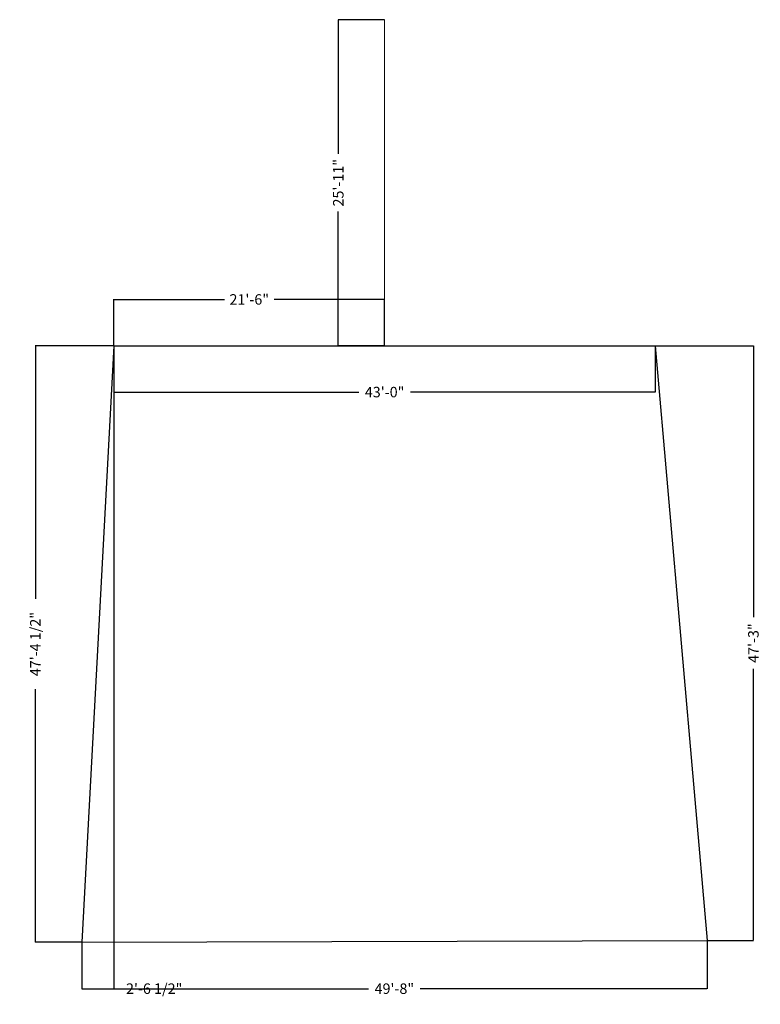
# Model space of a CAD drawing. Units: inches. Extents: x -269 to 4574, y -694 to 313.
# Tile 18 of 19: x 1868 to 2573, y -625 to 313. Entities that reach past the tile are written whole.
import ezdxf

# ---------------------------------------------------------------- set-up
doc = ezdxf.new("R2010")
doc.units = ezdxf.units.IN
doc.header["$MEASUREMENT"] = 0
for name, color, linetype, lineweight in [('C-PROP', 7, 'Continuous', 25), ('C-PROP-REFR', 8, 'Continuous', 13), ('DIMENSION', 5, 'Continuous', 18)]:
    doc.layers.add(name, color=color, linetype=linetype, lineweight=lineweight)
doc.dimstyles.get("Standard").update_dxf_attribs({"dimtxt": 10, "dimasz": 0.18, "dimexe": 0.18, "dimexo": 0.0625, "dimgap": 0.09, "dimtad": 0, "dimdec": 1, "dimzin": 0, "dimdsep": 46, "dimlunit": 3, "dimtxsty": 'Standard', "dimcen": 0.09, "dimclrt": 7, "dimadec": 0, "dimazin": 0, "dimtfac": 1, "dimtdec": 1, "dimtofl": 0, "dimtmove": 0, "dimatfit": 3, "dimfxl": 1, "dimtolj": 1, "dimtzin": 0, "dimarcsym": 0})

# ---------------------------------------------------------------- blocks, each defined once
blk = doc.blocks.new('*D67')
at = {"layer": 'Defpoints', "color": 0, "lineweight": 0, "transparency": 16777216}
for p in [(1926.59, -566.1), (2522.67, -564.28), (2522.67, -610.27)]:
    blk.add_point(p, dxfattribs=at)
at = {"layer": 'DIMENSION', "color": 0, "lineweight": -2, "transparency": 16777216}
for p, q in [((1926.59, -566.16), (1926.59, -610.45)), ((2522.67, -564.35), (2522.67, -610.45)), ((1926.77, -610.27), (2200.02, -610.27)), ((2522.49, -610.27), (2249.24, -610.27))]:
    blk.add_line(p, q, dxfattribs=at)
at = {"layer": 'DIMENSION', "color": 0, "lineweight": 0, "transparency": 16777216}
for points in [[(1926.77, -610.24), (1926.77, -610.3), (1926.59, -610.27)], [(2522.49, -610.24), (2522.49, -610.3), (2522.67, -610.27)]]:
    blk.add_solid(points, dxfattribs=at)
at = {"layer": 'DIMENSION', "color": 7, "transparency": 16777216, "insert": (2224.63, -610.27), "char_height": 10, "attachment_point": 5}
blk.add_mtext('\\A1;49\'-8"', dxfattribs=at)
blk = doc.blocks.new('*D68')
at = {"layer": 'Defpoints', "color": 0, "lineweight": 0, "transparency": 16777216}
for p in [(1957.34, 2.57), (2473.34, 2.57), (1957.34, -41.6)]:
    blk.add_point(p, dxfattribs=at)
at = {"layer": 'DIMENSION', "color": 0, "lineweight": -2, "transparency": 16777216}
for p, q in [((1957.34, 2.51), (1957.34, -41.78)), ((2473.34, 2.51), (2473.34, -41.78)), ((1957.52, -41.6), (2190.72, -41.6)), ((2473.16, -41.6), (2239.95, -41.6))]:
    blk.add_line(p, q, dxfattribs=at)
at = {"layer": 'DIMENSION', "color": 0, "lineweight": 0, "transparency": 16777216}
for points in [[(1957.52, -41.57), (1957.52, -41.63), (1957.34, -41.6)], [(2473.16, -41.57), (2473.16, -41.63), (2473.34, -41.6)]]:
    blk.add_solid(points, dxfattribs=at)
at = {"layer": 'DIMENSION', "color": 7, "transparency": 16777216, "insert": (2215.34, -41.6), "char_height": 10, "attachment_point": 5}
blk.add_mtext('\\A1;43\'-0"', dxfattribs=at)
blk = doc.blocks.new('*D69')
at = {"layer": 'Defpoints', "color": 0, "lineweight": 0, "transparency": 16777216}
for p in [(1882.42, 2.57), (1957.34, 2.57), (1926.59, -566.1)]:
    blk.add_point(p, dxfattribs=at)
at = {"layer": 'DIMENSION', "color": 0, "lineweight": -2, "transparency": 16777216}
for p, q in [((1957.27, 2.57), (1882.24, 2.57)), ((1882.42, 2.39), (1882.42, -238.81)), ((1882.42, -565.92), (1882.42, -324.71)), ((1926.53, -566.1), (1882.24, -566.1))]:
    blk.add_line(p, q, dxfattribs=at)
at = {"layer": 'DIMENSION', "color": 0, "lineweight": 0, "transparency": 16777216}
for points in [[(1882.39, 2.39), (1882.45, 2.39), (1882.42, 2.57)], [(1882.39, -565.92), (1882.45, -565.92), (1882.42, -566.1)]]:
    blk.add_solid(points, dxfattribs=at)
at = {"layer": 'DIMENSION', "color": 7, "transparency": 16777216, "insert": (1882.42, -281.76), "char_height": 10, "attachment_point": 5, "rotation": 90}
blk.add_mtext('\\A1;47\'-4 1/2"', dxfattribs=at)
blk = doc.blocks.new('*D70')
at = {"layer": 'Defpoints', "color": 0, "lineweight": 0, "transparency": 16777216}
for p in [(2473.34, 2.57), (2566.84, 2.57), (2522.67, -564.28)]:
    blk.add_point(p, dxfattribs=at)
at = {"layer": 'DIMENSION', "color": 0, "lineweight": -2, "transparency": 16777216}
for p, q in [((2473.4, 2.57), (2567.02, 2.57)), ((2566.84, 2.39), (2566.84, -256.24)), ((2566.84, -564.1), (2566.84, -305.47)), ((2522.73, -564.28), (2567.02, -564.28))]:
    blk.add_line(p, q, dxfattribs=at)
at = {"layer": 'DIMENSION', "color": 0, "lineweight": 0, "transparency": 16777216}
for points in [[(2566.81, 2.39), (2566.87, 2.39), (2566.84, 2.57)], [(2566.81, -564.1), (2566.87, -564.1), (2566.84, -564.28)]]:
    blk.add_solid(points, dxfattribs=at)
at = {"layer": 'DIMENSION', "color": 7, "transparency": 16777216, "insert": (2566.84, -280.85), "char_height": 10, "attachment_point": 5, "rotation": 90}
blk.add_mtext('\\A1;47\'-3"', dxfattribs=at)
blk = doc.blocks.new('*D71')
at = {"layer": 'Defpoints', "color": 0, "lineweight": 0, "transparency": 16777216}
for p in [(1957.34, 2.57), (1926.59, -566.1), (1957.34, -610.27)]:
    blk.add_point(p, dxfattribs=at)
at = {"layer": 'DIMENSION', "color": 0, "lineweight": -2, "transparency": 16777216}
for p, q in [((1957.34, 2.51), (1957.34, -610.45)), ((1926.59, -566.16), (1926.59, -610.45)), ((1926.77, -610.27), (1957.16, -610.27)), ((1957.34, -610.27), (1957.52, -610.27))]:
    blk.add_line(p, q, dxfattribs=at)
at = {"layer": 'DIMENSION', "color": 0, "lineweight": 0, "transparency": 16777216}
for points in [[(1926.77, -610.24), (1926.77, -610.3), (1926.59, -610.27)], [(1957.16, -610.24), (1957.16, -610.3), (1957.34, -610.27)]]:
    blk.add_solid(points, dxfattribs=at)
at = {"layer": 'DIMENSION', "color": 7, "transparency": 16777216, "insert": (1995.7, -610.27), "char_height": 10, "attachment_point": 5}
blk.add_mtext('\\A1;2\'-6 1/2"', dxfattribs=at)
blk = doc.blocks.new('*D72')
at = {"layer": 'Defpoints', "color": 0, "lineweight": 0, "transparency": 16777216}
for p in [(2215.34, 46.74), (1957.34, 2.57), (2215.34, 2.57)]:
    blk.add_point(p, dxfattribs=at)
at = {"layer": 'DIMENSION', "color": 0, "lineweight": -2, "transparency": 16777216}
for p, q in [((1957.34, 2.64), (1957.34, 46.92)), ((1957.52, 46.74), (2062.68, 46.74)), ((2215.16, 46.74), (2110, 46.74)), ((2215.34, 2.64), (2215.34, 46.92))]:
    blk.add_line(p, q, dxfattribs=at)
at = {"layer": 'DIMENSION', "color": 0, "lineweight": 0, "transparency": 16777216}
for points in [[(1957.52, 46.77), (1957.52, 46.71), (1957.34, 46.74)], [(2215.16, 46.77), (2215.16, 46.71), (2215.34, 46.74)]]:
    blk.add_solid(points, dxfattribs=at)
at = {"layer": 'DIMENSION', "color": 7, "transparency": 16777216, "insert": (2086.34, 46.74), "char_height": 10, "attachment_point": 5}
blk.add_mtext('\\A1;21\'-6"', dxfattribs=at)
blk = doc.blocks.new('*D73')
at = {"layer": 'Defpoints', "color": 0, "lineweight": 0, "transparency": 16777216}
for p in [(2171.17, 313.4), (2215.34, 313.4), (2215.34, 2.57)]:
    blk.add_point(p, dxfattribs=at)
at = {"layer": 'DIMENSION', "color": 0, "lineweight": -2, "transparency": 16777216}
for p, q in [((2215.27, 313.4), (2170.99, 313.4)), ((2171.17, 313.22), (2171.17, 185.46)), ((2171.17, 2.75), (2171.17, 130.51)), ((2215.27, 2.57), (2170.99, 2.57))]:
    blk.add_line(p, q, dxfattribs=at)
at = {"layer": 'DIMENSION', "color": 0, "lineweight": 0, "transparency": 16777216}
for points in [[(2171.14, 313.22), (2171.2, 313.22), (2171.17, 313.4)], [(2171.14, 2.75), (2171.2, 2.75), (2171.17, 2.57)]]:
    blk.add_solid(points, dxfattribs=at)
at = {"layer": 'DIMENSION', "color": 7, "transparency": 16777216, "insert": (2171.17, 157.99), "char_height": 10, "attachment_point": 5, "rotation": 90}
blk.add_mtext('\\A1;25\'-11"', dxfattribs=at)

msp = doc.modelspace()

# ---------------------------------------------------------------- linework, layer by layer
at = {"layer": 'C-PROP'}
for p, q in [((1957.34, 2.57), (1926.59, -566.1)), ((1957.34, 2.57), (2473.34, 2.57)), ((2473.34, 2.57), (2522.67, -564.28)), ((1926.59, -566.1), (2522.67, -564.28))]:
    msp.add_line(p, q, dxfattribs=at)
at = {"layer": 'C-PROP-REFR'}
msp.add_line((2215.34, 2.57), (2215.34, 313.4), dxfattribs=at)

# ---------------------------------------------------------------- dimensions: what is measured, and where the dimension line sits
at = {"layer": 'DIMENSION'}
for base, p1, p2, angle, picture, middle in [((2171.17, 313.4), (2215.34, 2.57), (2215.34, 313.4), 90, '*D73', (2171.17, 157.99)), ((1882.42, 2.57), (1926.59, -566.1), (1957.34, 2.57), 90, '*D69', (1882.42, -281.76)), ((1957.34, -41.6), (2473.34, 2.57), (1957.34, 2.57), 180, '*D68', (2215.34, -41.6)), ((2566.8395, 2.5737), (2522.6695, -564.2837), (2473.337, 2.5737), 90, '*D70', (2566.8395, -280.855))]:
    dim = msp.add_linear_dim(base=base, p1=p1, p2=p2, angle=angle, dimstyle='Standard', override={"dimdec": 1, "dimlfac": 1, "dimrnd": 0, "dimzin": 1, "dimdsep": 46, "dimlunit": 4, "dimfrac": 2}, dxfattribs=at)
    dim.commit()
    dim.dimension.update_dxf_attribs({"geometry": picture, "text_midpoint": middle})
for base, p1, p2, picture, middle in [((2215.34, 46.74), (1957.34, 2.57), (2215.34, 2.57), '*D72', (2086.34, 46.74)), ((1957.337, -610.2658), (1926.5922, -566.0958), (1957.337, 2.5737), '*D71', (1995.7022, -610.2658)), ((2522.67, -610.27), (1926.59, -566.1), (2522.67, -564.28), '*D67', (2224.63, -610.27))]:
    dim = msp.add_linear_dim(base=base, p1=p1, p2=p2, dimstyle='Standard', override={"dimdec": 1, "dimlfac": 1, "dimrnd": 0, "dimzin": 1, "dimdsep": 46, "dimlunit": 4, "dimfrac": 2}, dxfattribs=at)
    dim.commit()
    dim.dimension.update_dxf_attribs({"geometry": picture, "text_midpoint": middle})

doc.saveas('drawing.dxf')
